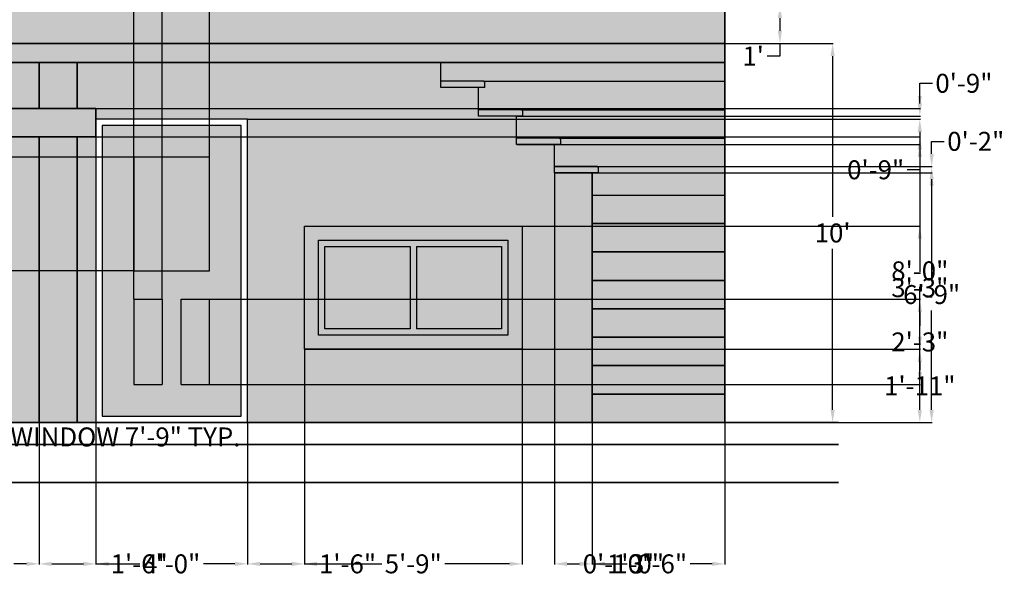
# Model space of a CAD drawing. Units: inches. Extents: x 23 to 640, y 58 to 516.
# Tile 3 of 4: x 328 to 640, y 67 to 243. Entities that reach past the tile are written whole.
import ezdxf

# ---------------------------------------------------------------- set-up
doc = ezdxf.new("R2010")
doc.units = ezdxf.units.IN
doc.header["$MEASUREMENT"] = 0
for name, color, linetype, lineweight in [('A-ANNO-DIMS', 2, 'Continuous', 18), ('A-DOOR', 3, 'Continuous', 25), ('A-ELEV', 7, 'Continuous', 35), ('A-ELEV-PATT', 252, 'Continuous', 13), ('A-FLOR-STRS', 7, 'Continuous', 25), ('A-GLAZ', 4, 'Continuous', 25)]:
    doc.layers.add(name, color=color, linetype=linetype, lineweight=lineweight)
doc.styles.get("Standard").update_dxf_attribs({"font": 'arial.ttf'})
doc.dimstyles.get("Standard").update_dxf_attribs({"dimtxt": 6, "dimasz": 4, "dimexe": 0.18, "dimexo": 0.0625, "dimgap": 2, "dimtad": 0, "dimtih": 1, "dimtoh": 1, "dimdec": 0, "dimzin": 0, "dimdsep": 46, "dimlunit": 3, "dimtxsty": 'Standard', "dimcen": 2, "dimadec": 0, "dimazin": 0, "dimtfac": 1, "dimtdec": 0, "dimtofl": 0, "dimtmove": 0, "dimatfit": 3, "dimfxl": 1, "dimtolj": 1, "dimtzin": 0, "dimarcsym": 0})

# ---------------------------------------------------------------- blocks, each defined once
blk = doc.blocks.new('*D9')
at = {"layer": 'A-ANNO-DIMS', "color": 0, "lineweight": -2, "transparency": 16777216}
for p, q in [((551.19, 247.68), (568.75, 247.68)), ((568.57, 243.68), (568.57, 239.68)), ((551.19, 235.68), (568.75, 235.68)), ((568.57, 235.68), (568.57, 231.68)), ((568.57, 231.68), (564.57, 231.68))]:
    blk.add_line(p, q, dxfattribs=at)
at = {"layer": 'A-ANNO-DIMS', "color": 0, "transparency": 16777216}
for points in [[(567.9, 243.68), (569.23, 243.68), (568.57, 247.68)], [(567.9, 239.68), (569.23, 239.68), (568.57, 235.68)]]:
    blk.add_solid(points, dxfattribs=at)
at = {"layer": 'Defpoints', "color": 0, "transparency": 16777216}
for p in [(551.13, 247.68), (551.13, 235.68), (568.57, 235.68)]:
    blk.add_point(p, dxfattribs=at)
at = {"layer": 'A-ANNO-DIMS', "color": 0, "transparency": 16777216, "insert": (560.09, 231.68), "char_height": 6, "attachment_point": 5}
blk.add_mtext("\\A1;1'", dxfattribs=at)
blk = doc.blocks.new('*D10')
at = {"layer": 'A-ANNO-DIMS', "color": 0, "lineweight": -2, "transparency": 16777216}
for p, q in [((551.19, 235.68), (585.45, 235.68)), ((585.27, 231.68), (585.27, 180.74)), ((585.27, 119.68), (585.27, 170.62)), ((551.19, 115.68), (585.45, 115.68))]:
    blk.add_line(p, q, dxfattribs=at)
at = {"layer": 'A-ANNO-DIMS', "color": 0, "transparency": 16777216}
for points in [[(584.6, 231.68), (585.93, 231.68), (585.27, 235.68)], [(584.6, 119.68), (585.93, 119.68), (585.27, 115.68)]]:
    blk.add_solid(points, dxfattribs=at)
at = {"layer": 'Defpoints', "color": 0, "transparency": 16777216}
for p in [(551.13, 235.68), (551.13, 115.68), (585.27, 115.68)]:
    blk.add_point(p, dxfattribs=at)
at = {"layer": 'A-ANNO-DIMS', "color": 0, "transparency": 16777216, "insert": (585.27, 175.68), "char_height": 6, "attachment_point": 5}
blk.add_mtext("\\A1;10'", dxfattribs=at)
blk = doc.blocks.new('*D15')
at = {"layer": 'A-ANNO-DIMS', "color": 0, "lineweight": -2, "transparency": 16777216}
for p, q in [((189.93, 125), (189.93, 110.93)), ((282.93, 125), (282.93, 110.93)), ((193.93, 111.11), (278.93, 111.11)), ((282.93, 111.11), (286.93, 111.11))]:
    blk.add_line(p, q, dxfattribs=at)
at = {"layer": 'A-ANNO-DIMS', "color": 0, "transparency": 16777216}
for points in [[(193.93, 111.78), (193.93, 110.44), (189.93, 111.11)], [(278.93, 111.78), (278.93, 110.44), (282.93, 111.11)]]:
    blk.add_solid(points, dxfattribs=at)
at = {"layer": 'Defpoints', "color": 0, "transparency": 16777216}
for p in [(189.93, 125.06), (282.93, 125.06), (282.93, 111.11)]:
    blk.add_point(p, dxfattribs=at)
at = {"layer": 'A-ANNO-DIMS', "color": 0, "transparency": 16777216, "insert": (344.69, 111.11), "char_height": 6, "attachment_point": 5}
blk.add_mtext('\\A1;SLIDING WINDOW 7\'-9" TYP.', dxfattribs=at)
blk = doc.blocks.new('*D26')
at = {"layer": 'A-ANNO-DIMS', "color": 0, "lineweight": -2, "transparency": 16777216}
for p, q in [((297.93, 115.62), (297.93, 70.75)), ((333.93, 115.62), (333.93, 70.75)), ((301.93, 70.93), (305.96, 70.93)), ((329.93, 70.93), (325.9, 70.93))]:
    blk.add_line(p, q, dxfattribs=at)
at = {"layer": 'A-ANNO-DIMS', "color": 0, "transparency": 16777216}
for points in [[(301.93, 71.6), (301.93, 70.26), (297.93, 70.93)], [(329.93, 71.6), (329.93, 70.26), (333.93, 70.93)]]:
    blk.add_solid(points, dxfattribs=at)
at = {"layer": 'Defpoints', "color": 0, "transparency": 16777216}
for p in [(297.93, 115.68), (333.93, 115.68), (333.93, 70.93)]:
    blk.add_point(p, dxfattribs=at)
at = {"layer": 'A-ANNO-DIMS', "color": 0, "transparency": 16777216, "insert": (315.93, 70.93), "char_height": 6, "attachment_point": 5}
blk.add_mtext('\\A1;3\'-0"', dxfattribs=at)
blk = doc.blocks.new('*D27')
at = {"layer": 'A-ANNO-DIMS', "color": 0, "lineweight": -2, "transparency": 16777216}
for p, q in [((333.93, 115.62), (333.93, 70.75)), ((351.93, 115.62), (351.93, 70.75)), ((337.93, 70.93), (347.93, 70.93)), ((351.93, 70.93), (355.93, 70.93))]:
    blk.add_line(p, q, dxfattribs=at)
at = {"layer": 'A-ANNO-DIMS', "color": 0, "transparency": 16777216}
for points in [[(337.93, 71.6), (337.93, 70.26), (333.93, 70.93)], [(347.93, 71.6), (347.93, 70.26), (351.93, 70.93)]]:
    blk.add_solid(points, dxfattribs=at)
at = {"layer": 'Defpoints', "color": 0, "transparency": 16777216}
for p in [(333.93, 115.68), (351.93, 115.68), (351.93, 70.93)]:
    blk.add_point(p, dxfattribs=at)
at = {"layer": 'A-ANNO-DIMS', "color": 0, "transparency": 16777216, "insert": (365.62, 70.93), "char_height": 6, "attachment_point": 5}
blk.add_mtext('\\A1;1\'-6"', dxfattribs=at)
blk = doc.blocks.new('*D28')
at = {"layer": 'A-ANNO-DIMS', "color": 0, "lineweight": -2, "transparency": 16777216}
for p, q in [((351.93, 115.62), (351.93, 70.75)), ((399.93, 115.62), (399.93, 70.75)), ((355.93, 70.93), (365.83, 70.93)), ((395.93, 70.93), (386.02, 70.93))]:
    blk.add_line(p, q, dxfattribs=at)
at = {"layer": 'A-ANNO-DIMS', "color": 0, "transparency": 16777216}
for points in [[(355.93, 71.6), (355.93, 70.26), (351.93, 70.93)], [(395.93, 71.6), (395.93, 70.26), (399.93, 70.93)]]:
    blk.add_solid(points, dxfattribs=at)
at = {"layer": 'Defpoints', "color": 0, "transparency": 16777216}
for p in [(351.93, 115.68), (399.93, 115.68), (399.93, 70.93)]:
    blk.add_point(p, dxfattribs=at)
at = {"layer": 'A-ANNO-DIMS', "color": 0, "transparency": 16777216, "insert": (375.93, 70.93), "char_height": 6, "attachment_point": 5}
blk.add_mtext('\\A1;4\'-0"', dxfattribs=at)
blk = doc.blocks.new('*D29')
at = {"layer": 'A-ANNO-DIMS', "color": 0, "lineweight": -2, "transparency": 16777216}
for p, q in [((417.93, 138.79), (417.93, 70.75)), ((399.93, 115.62), (399.93, 70.75)), ((403.93, 70.93), (413.93, 70.93)), ((417.93, 70.93), (421.93, 70.93))]:
    blk.add_line(p, q, dxfattribs=at)
at = {"layer": 'A-ANNO-DIMS', "color": 0, "transparency": 16777216}
for points in [[(403.93, 71.6), (403.93, 70.26), (399.93, 70.93)], [(413.93, 71.6), (413.93, 70.26), (417.93, 70.93)]]:
    blk.add_solid(points, dxfattribs=at)
at = {"layer": 'Defpoints', "color": 0, "transparency": 16777216}
for p in [(417.93, 138.86), (399.93, 115.68), (417.93, 70.93)]:
    blk.add_point(p, dxfattribs=at)
at = {"layer": 'A-ANNO-DIMS', "color": 0, "transparency": 16777216, "insert": (431.62, 70.93), "char_height": 6, "attachment_point": 5}
blk.add_mtext('\\A1;1\'-6"', dxfattribs=at)
blk = doc.blocks.new('*D30')
at = {"layer": 'A-ANNO-DIMS', "color": 0, "lineweight": -2, "transparency": 16777216}
for p, q in [((417.93, 138.79), (417.93, 70.75)), ((486.93, 138.79), (486.93, 70.75)), ((421.93, 70.93), (442.45, 70.93)), ((482.93, 70.93), (462.4, 70.93))]:
    blk.add_line(p, q, dxfattribs=at)
at = {"layer": 'A-ANNO-DIMS', "color": 0, "transparency": 16777216}
for points in [[(421.93, 71.6), (421.93, 70.26), (417.93, 70.93)], [(482.93, 71.6), (482.93, 70.26), (486.93, 70.93)]]:
    blk.add_solid(points, dxfattribs=at)
at = {"layer": 'Defpoints', "color": 0, "transparency": 16777216}
for p in [(417.93, 138.86), (486.93, 138.86), (486.93, 70.93)]:
    blk.add_point(p, dxfattribs=at)
at = {"layer": 'A-ANNO-DIMS', "color": 0, "transparency": 16777216, "insert": (452.43, 70.93), "char_height": 6, "attachment_point": 5}
blk.add_mtext('\\A1;5\'-9"', dxfattribs=at)
blk = doc.blocks.new('*D31')
at = {"layer": 'A-ANNO-DIMS', "color": 0, "lineweight": -2, "transparency": 16777216}
for p, q in [((497.13, 194.62), (497.13, 70.75)), ((486.93, 138.79), (486.93, 70.75)), ((482.93, 70.93), (478.93, 70.93)), ((501.13, 70.93), (505.13, 70.93))]:
    blk.add_line(p, q, dxfattribs=at)
at = {"layer": 'A-ANNO-DIMS', "color": 0, "transparency": 16777216}
for points in [[(482.93, 71.6), (482.93, 70.26), (486.93, 70.93)], [(501.13, 71.6), (501.13, 70.26), (497.13, 70.93)]]:
    blk.add_solid(points, dxfattribs=at)
at = {"layer": 'Defpoints', "color": 0, "transparency": 16777216}
for p in [(497.13, 194.68), (486.93, 138.86), (497.13, 70.93)]:
    blk.add_point(p, dxfattribs=at)
at = {"layer": 'A-ANNO-DIMS', "color": 0, "transparency": 16777216, "insert": (517.43, 70.93), "char_height": 6, "attachment_point": 5}
blk.add_mtext('\\A1;0\'-10"', dxfattribs=at)
blk = doc.blocks.new('*D32')
at = {"layer": 'A-ANNO-DIMS', "color": 0, "lineweight": -2, "transparency": 16777216}
for p, q in [((497.13, 194.62), (497.13, 70.75)), ((509.13, 194.62), (509.13, 70.75)), ((501.13, 70.93), (505.13, 70.93)), ((509.13, 70.93), (513.13, 70.93))]:
    blk.add_line(p, q, dxfattribs=at)
at = {"layer": 'A-ANNO-DIMS', "color": 0, "transparency": 16777216}
for points in [[(501.13, 71.6), (501.13, 70.26), (497.13, 70.93)], [(505.13, 71.6), (505.13, 70.26), (509.13, 70.93)]]:
    blk.add_solid(points, dxfattribs=at)
at = {"layer": 'Defpoints', "color": 0, "transparency": 16777216}
for p in [(497.13, 194.68), (509.13, 194.68), (509.13, 70.93)]:
    blk.add_point(p, dxfattribs=at)
at = {"layer": 'A-ANNO-DIMS', "color": 0, "transparency": 16777216, "insert": (522.82, 70.93), "char_height": 6, "attachment_point": 5}
blk.add_mtext('\\A1;1\'-0"', dxfattribs=at)
blk = doc.blocks.new('*D33')
at = {"layer": 'A-ANNO-DIMS', "color": 0, "lineweight": -2, "transparency": 16777216}
for p, q in [((509.13, 115.62), (509.13, 70.75)), ((551.13, 115.62), (551.13, 70.75)), ((513.13, 70.93), (520.16, 70.93)), ((547.13, 70.93), (540.1, 70.93))]:
    blk.add_line(p, q, dxfattribs=at)
at = {"layer": 'A-ANNO-DIMS', "color": 0, "transparency": 16777216}
for points in [[(513.13, 71.6), (513.13, 70.26), (509.13, 70.93)], [(547.13, 71.6), (547.13, 70.26), (551.13, 70.93)]]:
    blk.add_solid(points, dxfattribs=at)
at = {"layer": 'Defpoints', "color": 0, "transparency": 16777216}
for p in [(509.13, 115.68), (551.13, 115.68), (551.13, 70.93)]:
    blk.add_point(p, dxfattribs=at)
at = {"layer": 'A-ANNO-DIMS', "color": 0, "transparency": 16777216, "insert": (530.13, 70.93), "char_height": 6, "attachment_point": 5}
blk.add_mtext('\\A1;3\'-6"', dxfattribs=at)
blk = doc.blocks.new('*D35')
at = {"layer": 'A-ANNO-DIMS', "color": 0, "lineweight": -2, "transparency": 16777216}
for p, q in [((399.99, 211.68), (613.06, 211.68)), ((612.88, 207.68), (612.88, 168.74)), ((612.88, 119.68), (612.88, 158.62)), ((399.99, 115.68), (613.06, 115.68))]:
    blk.add_line(p, q, dxfattribs=at)
at = {"layer": 'A-ANNO-DIMS', "color": 0, "transparency": 16777216}
for points in [[(612.21, 207.68), (613.55, 207.68), (612.88, 211.68)], [(612.21, 119.68), (613.55, 119.68), (612.88, 115.68)]]:
    blk.add_solid(points, dxfattribs=at)
at = {"layer": 'Defpoints', "color": 0, "transparency": 16777216}
for p in [(399.93, 211.68), (612.88, 211.68), (399.93, 115.68)]:
    blk.add_point(p, dxfattribs=at)
at = {"layer": 'A-ANNO-DIMS', "color": 0, "transparency": 16777216, "insert": (612.88, 163.68), "char_height": 6, "attachment_point": 5}
blk.add_mtext('\\A1;8\'-0"', dxfattribs=at)
blk = doc.blocks.new('*D36')
at = {"layer": 'A-ANNO-DIMS', "color": 0, "lineweight": -2, "transparency": 16777216}
for p, q in [((359.93, 507.43), (355.93, 507.43)), ((363.93, 163.74), (363.93, 507.61)), ((387.93, 199.74), (387.93, 507.61)), ((391.93, 507.43), (395.93, 507.43))]:
    blk.add_line(p, q, dxfattribs=at)
at = {"layer": 'A-ANNO-DIMS', "color": 0, "transparency": 16777216}
for points in [[(359.93, 508.1), (359.93, 506.76), (363.93, 507.43)], [(391.93, 508.1), (391.93, 506.76), (387.93, 507.43)]]:
    blk.add_solid(points, dxfattribs=at)
at = {"layer": 'Defpoints', "color": 0, "transparency": 16777216}
for p in [(387.93, 507.43), (387.93, 199.68), (363.93, 163.68)]:
    blk.add_point(p, dxfattribs=at)
at = {"layer": 'A-ANNO-DIMS', "color": 0, "transparency": 16777216, "insert": (375.93, 507.43), "char_height": 6, "attachment_point": 5}
blk.add_mtext('\\A1;2\'-0"', dxfattribs=at)
blk = doc.blocks.new('*D37')
at = {"layer": 'A-ANNO-DIMS', "color": 0, "lineweight": -2, "transparency": 16777216}
for p, q in [((363.87, 199.68), (63.5, 199.68)), ((63.68, 195.68), (63.68, 186.75)), ((63.68, 167.68), (63.68, 176.62)), ((363.87, 163.68), (63.5, 163.68))]:
    blk.add_line(p, q, dxfattribs=at)
at = {"layer": 'A-ANNO-DIMS', "color": 0, "transparency": 16777216}
for points in [[(63.01, 195.68), (64.35, 195.68), (63.68, 199.68)], [(63.01, 167.68), (64.35, 167.68), (63.68, 163.68)]]:
    blk.add_solid(points, dxfattribs=at)
at = {"layer": 'Defpoints', "color": 0, "transparency": 16777216}
for p in [(63.68, 199.68), (363.93, 199.68), (363.93, 163.68)]:
    blk.add_point(p, dxfattribs=at)
at = {"layer": 'A-ANNO-DIMS', "color": 0, "transparency": 16777216, "insert": (63.68, 181.68), "char_height": 6, "attachment_point": 5}
blk.add_mtext('\\A1;3\'-0"', dxfattribs=at)
blk = doc.blocks.new('*D38')
at = {"layer": 'A-ANNO-DIMS', "color": 0, "lineweight": -2, "transparency": 16777216}
for p, q in [((359.93, 507.43), (355.93, 507.43)), ((363.93, 154.74), (363.93, 507.61)), ((372.93, 154.74), (372.93, 507.61)), ((376.93, 507.43), (380.93, 507.43))]:
    blk.add_line(p, q, dxfattribs=at)
at = {"layer": 'A-ANNO-DIMS', "color": 0, "transparency": 16777216}
for points in [[(359.93, 508.1), (359.93, 506.76), (363.93, 507.43)], [(376.93, 508.1), (376.93, 506.76), (372.93, 507.43)]]:
    blk.add_solid(points, dxfattribs=at)
at = {"layer": 'Defpoints', "color": 0, "transparency": 16777216}
for p in [(372.93, 507.43), (363.93, 154.68), (372.93, 154.68)]:
    blk.add_point(p, dxfattribs=at)
at = {"layer": 'A-ANNO-DIMS', "color": 0, "transparency": 16777216, "insert": (390.9, 507.43), "char_height": 6, "attachment_point": 5}
blk.add_mtext('\\A1;0\'-9"', dxfattribs=at)
blk = doc.blocks.new('*D39')
at = {"layer": 'A-ANNO-DIMS', "color": 0, "lineweight": -2, "transparency": 16777216}
for p, q in [((387.99, 154.68), (613.06, 154.68)), ((612.88, 150.68), (612.88, 146.25)), ((612.88, 131.68), (612.88, 136.12)), ((387.99, 127.68), (613.06, 127.68))]:
    blk.add_line(p, q, dxfattribs=at)
at = {"layer": 'A-ANNO-DIMS', "color": 0, "transparency": 16777216}
for points in [[(612.21, 150.68), (613.55, 150.68), (612.88, 154.68)], [(612.21, 131.68), (613.55, 131.68), (612.88, 127.68)]]:
    blk.add_solid(points, dxfattribs=at)
at = {"layer": 'Defpoints', "color": 0, "transparency": 16777216}
for p in [(387.93, 154.68), (612.88, 154.68), (387.93, 127.68)]:
    blk.add_point(p, dxfattribs=at)
at = {"layer": 'A-ANNO-DIMS', "color": 0, "transparency": 16777216, "insert": (612.88, 141.18), "char_height": 6, "attachment_point": 5}
blk.add_mtext('\\A1;2\'-3"', dxfattribs=at)
blk = doc.blocks.new('*D40')
at = {"layer": 'A-ANNO-DIMS', "color": 0, "lineweight": -2, "transparency": 16777216}
for p, q in [((417.99, 138.86), (613.06, 138.86)), ((612.88, 134.86), (612.88, 132.28)), ((612.88, 119.68), (612.88, 122.26)), ((399.99, 115.68), (613.06, 115.68))]:
    blk.add_line(p, q, dxfattribs=at)
at = {"layer": 'A-ANNO-DIMS', "color": 0, "transparency": 16777216}
for points in [[(612.21, 134.86), (613.55, 134.86), (612.88, 138.86)], [(612.21, 119.68), (613.55, 119.68), (612.88, 115.68)]]:
    blk.add_solid(points, dxfattribs=at)
at = {"layer": 'Defpoints', "color": 0, "transparency": 16777216}
for p in [(417.93, 138.86), (612.88, 138.86), (399.93, 115.68)]:
    blk.add_point(p, dxfattribs=at)
at = {"layer": 'A-ANNO-DIMS', "color": 0, "transparency": 16777216, "insert": (612.88, 127.27), "char_height": 6, "attachment_point": 5}
blk.add_mtext('\\A1;1\'-11"', dxfattribs=at)
blk = doc.blocks.new('*D41')
at = {"layer": 'A-ANNO-DIMS', "color": 0, "lineweight": -2, "transparency": 16777216}
for p, q in [((486.99, 177.86), (613.06, 177.86)), ((612.88, 173.86), (612.88, 163.42)), ((612.88, 142.86), (612.88, 153.29)), ((486.99, 138.86), (613.06, 138.86))]:
    blk.add_line(p, q, dxfattribs=at)
at = {"layer": 'A-ANNO-DIMS', "color": 0, "transparency": 16777216}
for points in [[(612.21, 173.86), (613.55, 173.86), (612.88, 177.86)], [(612.21, 142.86), (613.55, 142.86), (612.88, 138.86)]]:
    blk.add_solid(points, dxfattribs=at)
at = {"layer": 'Defpoints', "color": 0, "transparency": 16777216}
for p in [(486.93, 177.86), (612.88, 177.86), (486.93, 138.86)]:
    blk.add_point(p, dxfattribs=at)
at = {"layer": 'A-ANNO-DIMS', "color": 0, "transparency": 16777216, "insert": (612.88, 158.36), "char_height": 6, "attachment_point": 5}
blk.add_mtext('\\A1;3\'-3"', dxfattribs=at)
blk = doc.blocks.new('*D46')
at = {"layer": 'A-ANNO-DIMS', "color": 0, "lineweight": -2, "transparency": 16777216}
for p, q in [((612.88, 216.68), (612.88, 220.68)), ((485.19, 212.68), (613.06, 212.68)), ((485.19, 203.68), (613.06, 203.68)), ((612.88, 199.68), (612.88, 195.68)), ((612.88, 195.68), (608.88, 195.68))]:
    blk.add_line(p, q, dxfattribs=at)
at = {"layer": 'A-ANNO-DIMS', "color": 0, "transparency": 16777216}
for points in [[(612.21, 216.68), (613.55, 216.68), (612.88, 212.68)], [(612.21, 199.68), (613.55, 199.68), (612.88, 203.68)]]:
    blk.add_solid(points, dxfattribs=at)
at = {"layer": 'Defpoints', "color": 0, "transparency": 16777216}
for p in [(485.13, 212.68), (485.13, 203.68), (612.88, 203.68)]:
    blk.add_point(p, dxfattribs=at)
at = {"layer": 'A-ANNO-DIMS', "color": 0, "transparency": 16777216, "insert": (598.9, 195.68), "char_height": 6, "attachment_point": 5}
blk.add_mtext('\\A1;0\'-9"', dxfattribs=at)
blk = doc.blocks.new('*D47')
at = {"layer": 'A-ANNO-DIMS', "color": 0, "lineweight": -2, "transparency": 16777216}
for p, q in [((612.88, 219.06), (612.88, 223.06)), ((612.88, 223.06), (616.88, 223.06)), ((351.99, 215.06), (613.06, 215.06)), ((351.99, 206.06), (613.06, 206.06)), ((612.88, 202.06), (612.88, 198.06))]:
    blk.add_line(p, q, dxfattribs=at)
at = {"layer": 'A-ANNO-DIMS', "color": 0, "transparency": 16777216}
for points in [[(612.21, 219.06), (613.55, 219.06), (612.88, 215.06)], [(612.21, 202.06), (613.55, 202.06), (612.88, 206.06)]]:
    blk.add_solid(points, dxfattribs=at)
at = {"layer": 'Defpoints', "color": 0, "transparency": 16777216}
for p in [(351.93, 215.06), (612.88, 215.06), (351.93, 206.06)]:
    blk.add_point(p, dxfattribs=at)
at = {"layer": 'A-ANNO-DIMS', "color": 0, "transparency": 16777216, "insert": (626.85, 223.06), "char_height": 6, "attachment_point": 5}
blk.add_mtext('\\A1;0\'-9"', dxfattribs=at)
blk = doc.blocks.new('*D50')
at = {"layer": 'A-ANNO-DIMS', "color": 0, "lineweight": -2, "transparency": 16777216}
for p, q in [((510.69, 196.68), (616.81, 196.68)), ((616.63, 192.68), (616.63, 161.24)), ((616.63, 119.68), (616.63, 151.12)), ((509.19, 115.68), (616.81, 115.68))]:
    blk.add_line(p, q, dxfattribs=at)
at = {"layer": 'A-ANNO-DIMS', "color": 0, "transparency": 16777216}
for points in [[(615.96, 192.68), (617.3, 192.68), (616.63, 196.68)], [(615.96, 119.68), (617.3, 119.68), (616.63, 115.68)]]:
    blk.add_solid(points, dxfattribs=at)
at = {"layer": 'Defpoints', "color": 0, "transparency": 16777216}
for p in [(510.63, 196.68), (616.63, 196.68), (509.13, 115.68)]:
    blk.add_point(p, dxfattribs=at)
at = {"layer": 'A-ANNO-DIMS', "color": 0, "transparency": 16777216, "insert": (616.63, 156.18), "char_height": 6, "attachment_point": 5}
blk.add_mtext('\\A1;6\'-9"', dxfattribs=at)
blk = doc.blocks.new('*D51')
at = {"layer": 'A-ANNO-DIMS', "color": 0, "lineweight": -2, "transparency": 16777216}
for p, q in [((616.63, 200.68), (616.63, 204.68)), ((616.63, 204.68), (620.63, 204.68)), ((497.19, 196.68), (616.81, 196.68)), ((497.19, 194.68), (616.81, 194.68)), ((616.63, 190.68), (616.63, 186.68))]:
    blk.add_line(p, q, dxfattribs=at)
at = {"layer": 'A-ANNO-DIMS', "color": 0, "transparency": 16777216}
for points in [[(615.96, 200.68), (617.3, 200.68), (616.63, 196.68)], [(615.96, 190.68), (617.3, 190.68), (616.63, 194.68)]]:
    blk.add_solid(points, dxfattribs=at)
at = {"layer": 'Defpoints', "color": 0, "transparency": 16777216}
for p in [(497.13, 196.68), (616.63, 196.68), (497.13, 194.68)]:
    blk.add_point(p, dxfattribs=at)
at = {"layer": 'A-ANNO-DIMS', "color": 0, "transparency": 16777216, "insert": (630.6, 204.68), "char_height": 6, "attachment_point": 5}
blk.add_mtext('\\A1;0\'-2"', dxfattribs=at)

msp = doc.modelspace()

# ---------------------------------------------------------------- hatches: boundary and pattern name
at = {"layer": 'A-ELEV-PATT'}
h = msp.add_hatch(color=256, dxfattribs=at)
h.dxf.hatch_style = 1
h.paths.add_polyline_path([(333.93, 433.68), (297.93, 433.68), (297.93, 379.68), (333.93, 379.68)])
h.paths.add_polyline_path([(333.93, 379.68), (297.93, 379.68), (297.93, 367.68), (333.93, 367.68)])
h.paths.add_polyline_path([(333.93, 358.68), (297.93, 358.68), (297.93, 247.68), (333.93, 247.68)])
h.paths.add_polyline_path([(333.93, 229.68), (297.93, 229.68), (297.93, 215.06), (333.93, 215.06)])
h.paths.add_polyline_path([(333.93, 206.06), (297.93, 206.06), (297.93, 115.68), (333.93, 115.68)])
h = msp.add_hatch(color=256, dxfattribs=at)
h.dxf.hatch_style = 1
h.paths.add_polyline_path([(371.93, 367.68), (180.93, 367.68), (180.93, 247.68), (189.93, 247.68), (189.93, 358.68), (371.93, 358.68)])
h.paths.add_polyline_path([(189.93, 247.68), (180.93, 247.68), (180.93, 235.68), (189.93, 235.68)])
h.paths.add_polyline_path([(189.93, 235.68), (180.93, 235.68), (180.93, 206.06), (333.93, 206.06), (351.93, 206.06), (351.93, 211.68), (351.93, 215.06), (189.93, 215.06)])
h.paths.add_polyline_path([(551.13, 247.68), (280.13, 247.68), (280.13, 235.68), (551.13, 235.68)])
h.paths.add_polyline_path([(551.13, 235.68), (280.13, 235.68), (280.13, 229.68), (551.13, 229.68)])
h = msp.add_hatch(color=256, dxfattribs=at)
h.set_gradient(color1=(147, 149, 152), color2=(199, 200, 202), name='INVCYLINDER')
h.paths.add_polyline_path([(333.93, 215.06), (345.93, 215.06), (345.93, 229.68), (333.93, 229.68)])
h = msp.add_hatch(color=256, dxfattribs=at)
h.set_gradient(color1=(255, 255, 255), color2=(147, 149, 152), name='INVHEMISPHERICAL')
h.paths.add_polyline_path([(399.93, 115.68), (509.13, 115.68), (509.13, 187.68), (509.13, 194.68), (497.13, 194.68), (497.13, 203.68), (485.13, 203.68), (485.13, 212.68), (473.13, 212.68), (473.13, 221.68), (461.13, 221.68), (461.13, 229.68), (345.93, 229.68), (345.93, 215.06), (351.93, 215.06), (351.93, 211.68), (399.93, 211.68)])
h.paths.add_polyline_path([(486.93, 177.86), (486.93, 138.86), (417.93, 138.86), (417.93, 177.86)], flags=16)
h.paths.add_polyline_path([(482.43, 173.36), (482.43, 143.36), (422.43, 143.36), (422.43, 173.36)], flags=0)
h.paths.add_polyline_path([(451.43, 171.36), (451.43, 145.36), (424.43, 145.36), (424.43, 171.36)], flags=0)
h.paths.add_polyline_path([(453.43, 171.36), (480.43, 171.36), (480.43, 145.36), (453.43, 145.36)], flags=0)
h = msp.add_hatch(color=256, dxfattribs=at)
h.set_gradient(color1=(206, 204, 230), color2=(99, 100, 102), name='INVHEMISPHERICAL')
h.paths.add_polyline_path([(551.13, 229.68), (461.13, 229.68), (461.13, 223.68), (474.63, 223.68), (551.13, 223.68)])
h.paths.add_polyline_path([(551.13, 223.68), (474.63, 223.68, -0.414214), (475.13, 223.18), (475.13, 221.68), (473.13, 221.68), (473.13, 214.68), (486.63, 214.68), (551.13, 214.68)])
h.paths.add_polyline_path([(551.13, 214.68), (486.63, 214.68, -0.414214), (487.13, 214.18), (487.13, 212.68), (485.13, 212.68), (485.13, 205.68), (498.63, 205.68), (551.13, 205.68)])
h.paths.add_polyline_path([(551.13, 205.68), (498.63, 205.68, -0.414214), (499.13, 205.18), (499.13, 203.68), (497.13, 203.68), (497.13, 196.68), (510.63, 196.68), (551.13, 196.68)])
h.paths.add_polyline_path([(551.13, 196.68), (510.63, 196.68, -0.414214), (511.13, 196.18), (511.13, 194.68), (509.13, 194.68), (509.13, 187.68), (551.13, 187.68)])
h = msp.add_hatch(color=256, dxfattribs=at)
h.set_gradient(color1=(255, 255, 255), color2=(147, 149, 152))
h.paths.add_polyline_path([(461.13, 223.68), (461.13, 221.68), (475.13, 221.68), (475.13, 223.18, 0.414214), (474.63, 223.68)])
h.paths.add_polyline_path([(487.13, 212.68), (487.13, 214.18, 0.414214), (486.63, 214.68), (473.13, 214.68), (473.13, 212.68)])
h.paths.add_polyline_path([(499.13, 203.68), (499.13, 205.18, 0.414214), (498.63, 205.68), (485.13, 205.68), (485.13, 203.68)])
h.paths.add_polyline_path([(497.13, 196.68), (497.13, 194.68), (511.13, 194.68), (511.13, 196.18, 0.414214), (510.63, 196.68)])
h = msp.add_hatch(color=256, dxfattribs=at)
h.set_gradient(color1=(255, 255, 255), color2=(147, 149, 152), name='SPHERICAL')
h.paths.add_polyline_path([(353.93, 117.68), (397.93, 117.68), (397.93, 209.68), (353.93, 209.68)])
h.paths.add_polyline_path([(363.93, 163.68), (363.93, 199.68), (387.93, 199.68), (387.93, 163.68)], flags=16)
h.paths.add_polyline_path([(363.93, 154.68), (372.93, 154.68), (372.93, 127.68), (363.93, 127.68)], flags=16)
h.paths.add_polyline_path([(378.93, 154.68), (387.93, 154.68), (387.93, 127.68), (378.93, 127.68)], flags=16)
h = msp.add_hatch(color=256, dxfattribs=at)
h.set_gradient(color1=(147, 149, 152), color2=(199, 200, 202), name='INVCYLINDER')
h.paths.add_polyline_path([(345.93, 206.06), (333.93, 206.06), (333.93, 115.68), (345.93, 115.68)])
h = msp.add_hatch(color=256, dxfattribs=at)
h.set_gradient(color1=(255, 255, 255), color2=(147, 149, 152), name='CYLINDER')
h.paths.add_polyline_path([(345.93, 115.68), (351.93, 115.68), (351.93, 206.06), (345.93, 206.06)])
h = msp.add_hatch(color=256, dxfattribs=at)
h.set_gradient(color1=(99, 100, 102), color2=(147, 149, 152), name='CYLINDER')
h.paths.add_polyline_path([(363.93, 163.68), (387.93, 163.68), (387.93, 199.68), (363.93, 199.68)])
h = msp.add_hatch(color=256, dxfattribs=at)
h.set_gradient(color1=(199, 200, 202), color2=(147, 149, 152), name='CYLINDER')
h.paths.add_polyline_path([(509.13, 187.68), (509.13, 178.68), (551.13, 178.68), (551.13, 187.68)])
h = msp.add_hatch(color=256, dxfattribs=at)
h.set_gradient(color1=(153, 76, 76), color2=(147, 149, 152), name='SPHERICAL')
h.paths.add_polyline_path([(417.93, 177.86), (417.93, 138.86), (486.93, 138.86), (486.93, 177.86)])
h.paths.add_polyline_path([(422.43, 173.36), (482.43, 173.36), (482.43, 143.36), (422.43, 143.36)], flags=16)
h.paths.add_polyline_path([(424.43, 171.36), (451.43, 171.36), (451.43, 145.36), (424.43, 145.36)], flags=0)
h.paths.add_polyline_path([(453.43, 171.36), (480.43, 171.36), (480.43, 145.36), (453.43, 145.36)], flags=0)
h = msp.add_hatch(color=256, dxfattribs=at)
h.set_gradient(color1=(147, 149, 152), color2=(199, 200, 202), name='CYLINDER')
h.paths.add_polyline_path([(551.13, 169.68), (551.13, 178.68), (509.13, 178.68), (509.13, 169.68)])
h = msp.add_hatch(color=256, dxfattribs=at)
h.set_gradient(color1=(99, 100, 102), color2=(66, 66, 66), name='SPHERICAL')
h.paths.add_polyline_path([(422.43, 173.36), (422.43, 143.36), (482.43, 143.36), (482.43, 173.36)])
h.paths.add_polyline_path([(424.43, 171.36), (451.43, 171.36), (451.43, 145.36), (424.43, 145.36)], flags=16)
h.paths.add_polyline_path([(453.43, 171.36), (480.43, 171.36), (480.43, 145.36), (453.43, 145.36)], flags=16)
h = msp.add_hatch(color=256, dxfattribs=at)
h.set_gradient(color1=(255, 255, 255), color2=(173, 221, 247), name='INVSPHERICAL')
h.paths.add_polyline_path([(451.43, 171.36), (424.43, 171.36), (424.43, 145.36), (451.43, 145.36)])
h = msp.add_hatch(color=256, dxfattribs=at)
h.set_gradient(color1=(255, 255, 255), color2=(173, 221, 247), name='INVSPHERICAL')
h.paths.add_polyline_path([(480.43, 145.36), (480.43, 171.36), (453.43, 171.36), (453.43, 145.36)])
h = msp.add_hatch(color=256, dxfattribs=at)
h.set_gradient(color1=(199, 200, 202), color2=(147, 149, 152), name='CYLINDER')
h.paths.add_polyline_path([(509.13, 169.68), (509.13, 160.68), (551.13, 160.68), (551.13, 169.68)])
h = msp.add_hatch(color=256, dxfattribs=at)
h.set_gradient(color1=(147, 149, 152), color2=(199, 200, 202), name='CYLINDER')
h.paths.add_polyline_path([(509.13, 160.68), (509.13, 151.68), (551.13, 151.68), (551.13, 160.68)])
h = msp.add_hatch(color=256, dxfattribs=at)
h.set_gradient(color1=(99, 100, 102), color2=(147, 149, 152), name='CYLINDER')
h.paths.add_polyline_path([(372.93, 154.68), (363.93, 154.68), (363.93, 127.68), (372.93, 127.68)])
h = msp.add_hatch(color=256, dxfattribs=at)
h.set_gradient(color1=(99, 100, 102), color2=(147, 149, 152), name='CYLINDER')
h.paths.add_polyline_path([(378.93, 127.68), (387.93, 127.68), (387.93, 154.68), (378.93, 154.68)])
h = msp.add_hatch(color=256, dxfattribs=at)
h.set_gradient(color1=(199, 200, 202), color2=(147, 149, 152), name='CYLINDER')
h.paths.add_polyline_path([(551.13, 142.68), (551.13, 151.68), (509.13, 151.68), (509.13, 142.68)])
h = msp.add_hatch(color=256, dxfattribs=at)
h.set_gradient(color1=(147, 149, 152), color2=(199, 200, 202), name='CYLINDER')
h.paths.add_polyline_path([(509.13, 142.68), (509.13, 133.68), (551.13, 133.68), (551.13, 142.68)])
h = msp.add_hatch(color=256, dxfattribs=at)
h.set_gradient(color1=(199, 200, 202), color2=(147, 149, 152), name='CYLINDER')
h.paths.add_polyline_path([(551.13, 124.68), (551.13, 133.68), (509.13, 133.68), (509.13, 124.68)])
h = msp.add_hatch(color=256, dxfattribs=at)
h.set_gradient(color1=(147, 149, 152), color2=(199, 200, 202), name='CYLINDER')
h.paths.add_polyline_path([(509.13, 124.68), (509.13, 115.68), (551.13, 115.68), (551.13, 124.68)])

# ---------------------------------------------------------------- linework, layer by layer
at = {"layer": 'A-DOOR'}
for p, q in [((387.93, 199.68), (363.93, 199.68)), ((363.93, 199.68), (363.93, 163.68)), ((387.93, 163.68), (387.93, 199.68)), ((363.93, 163.68), (387.93, 163.68)), ((363.93, 154.68), (372.93, 154.68)), ((363.93, 154.68), (363.93, 127.68)), ((372.93, 154.68), (372.93, 127.68)), ((378.93, 127.68), (378.93, 154.68)), ((378.93, 154.68), (387.93, 154.68)), ((387.93, 127.68), (387.93, 154.68)), ((363.93, 127.68), (372.93, 127.68)), ((378.93, 127.68), (387.93, 127.68))]:
    msp.add_line(p, q, dxfattribs=at)
for points in [[(351.93, 115.68), (399.93, 115.68), (399.93, 211.68), (351.93, 211.68)], [(353.93, 117.68), (397.93, 117.68), (397.93, 209.68), (353.93, 209.68)]]:
    msp.add_lwpolyline(points, close=True, dxfattribs=at)
at = {"layer": 'A-ELEV'}
for p, q in [((551.13, 379.68), (551.13, 115.68)), ((125.43, 235.68), (551.13, 235.68)), ((280.13, 229.68), (551.13, 229.68)), ((333.93, 229.68), (333.93, 215.06)), ((345.93, 229.68), (345.93, 215.06)), ((351.93, 215.06), (189.93, 215.06)), ((351.93, 206.06), (351.93, 215.06)), ((180.93, 206.06), (333.93, 206.06)), ((333.93, 206.06), (351.93, 206.06)), ((333.93, 206.06), (333.93, 115.68)), ((345.93, 206.06), (345.93, 115.68)), ((509.13, 187.68), (509.13, 115.68)), ((509.13, 178.68), (551.13, 178.68)), ((509.13, 169.68), (551.13, 169.68)), ((509.13, 160.68), (551.13, 160.68)), ((509.13, 151.68), (551.13, 151.68)), ((509.13, 142.68), (551.13, 142.68)), ((509.13, 133.68), (551.13, 133.68)), ((509.13, 124.68), (551.13, 124.68)), ((89.43, 115.68), (587.13, 115.68)), ((89.43, 108.68), (587.13, 108.68)), ((89.43, 96.68), (587.13, 96.68))]:
    msp.add_line(p, q, dxfattribs=at)
at = {"layer": 'A-FLOR-STRS'}
for p, q in [((461.13, 221.68), (461.13, 229.68)), ((474.63, 223.68), (461.13, 223.68)), ((475.13, 221.68), (461.13, 221.68)), ((473.13, 212.68), (473.13, 221.68)), ((474.63, 223.68), (551.13, 223.68)), ((475.13, 221.68), (475.13, 223.18)), ((486.63, 214.68), (473.13, 214.68)), ((487.13, 212.68), (473.13, 212.68)), ((485.13, 203.68), (485.13, 212.68)), ((486.63, 214.68), (551.13, 214.68)), ((487.13, 212.68), (487.13, 214.18)), ((498.63, 205.68), (485.13, 205.68)), ((499.13, 203.68), (485.13, 203.68)), ((497.13, 194.68), (497.13, 203.68)), ((498.63, 205.68), (551.13, 205.68)), ((499.13, 203.68), (499.13, 205.18)), ((510.63, 196.68), (497.13, 196.68)), ((510.63, 196.68), (551.13, 196.68)), ((511.13, 194.68), (497.13, 194.68)), ((509.13, 187.68), (509.13, 194.68)), ((511.13, 194.68), (511.13, 196.18)), ((509.13, 187.68), (551.13, 187.68))]:
    msp.add_line(p, q, dxfattribs=at)
for centre in [(474.63, 223.18), (486.63, 214.18), (498.63, 205.18), (510.63, 196.18)]:
    msp.add_arc(centre, 0.5, 0, 90, dxfattribs=at)
at = {"layer": 'A-GLAZ'}
for p, q in [((451.43, 171.36), (451.43, 145.36)), ((453.43, 171.36), (453.43, 145.36))]:
    msp.add_line(p, q, dxfattribs=at)
for points in [[(417.93, 177.86), (486.93, 177.86), (486.93, 138.86), (417.93, 138.86)], [(422.43, 173.36), (482.43, 173.36), (482.43, 143.36), (422.43, 143.36)]]:
    msp.add_lwpolyline(points, close=True, dxfattribs=at)
for points in [[(451.43, 145.36), (424.43, 145.36), (424.43, 171.36), (451.43, 171.36)], [(453.43, 171.36), (480.43, 171.36), (480.43, 145.36), (453.43, 145.36)]]:
    msp.add_lwpolyline(points, dxfattribs=at)

# ---------------------------------------------------------------- dimensions: what is measured, and where the dimension line sits
at = {"layer": 'A-ANNO-DIMS'}
for base, p1, p2, picture, middle in [((387.93, 507.43), (363.93, 163.68), (387.93, 199.68), '*D36', (375.93, 507.43)), ((372.93, 507.43), (363.93, 154.68), (372.93, 154.68), '*D38', (390.9, 507.43)), ((497.13, 70.93), (486.93, 138.86), (497.13, 194.68), '*D31', (517.43, 70.93)), ((509.13, 70.93), (497.13, 194.68), (509.13, 194.68), '*D32', (522.82, 70.93)), ((417.93, 70.93), (399.93, 115.68), (417.93, 138.86), '*D29', (431.62, 70.93)), ((486.93, 70.93), (417.93, 138.86), (486.93, 138.86), '*D30', (452.43, 70.93)), ((333.93, 70.93), (297.93, 115.68), (333.93, 115.68), '*D26', (315.93, 70.93)), ((351.93, 70.93), (333.93, 115.68), (351.93, 115.68), '*D27', (365.62, 70.93)), ((399.93, 70.93), (351.93, 115.68), (399.93, 115.68), '*D28', (375.93, 70.93)), ((551.13, 70.93), (509.13, 115.68), (551.13, 115.68), '*D33', (530.13, 70.93))]:
    dim = msp.add_linear_dim(base=base, p1=p1, p2=p2, dimstyle='Standard', override={"dimdec": 1, "dimlfac": 1, "dimrnd": 0, "dimzin": 1, "dimdsep": 46, "dimlunit": 4, "dimfrac": 2}, dxfattribs=at)
    dim.commit()
    dim.dimension.update_dxf_attribs({"geometry": picture, "text_midpoint": middle})
for base, p1, p2, override, picture, middle in [((568.57, 235.68), (551.13, 247.68), (551.13, 235.68), {"dimclrd": 0, "dimclre": 0, "dimclrt": 0}, '*D9', (560.09, 231.68)), ((585.27, 115.68), (551.13, 235.68), (551.13, 115.68), {"dimclrd": 0, "dimclre": 0, "dimclrt": 0}, '*D10', (585.27, 175.68)), ((612.88, 215.06), (351.93, 206.06), (351.93, 215.06), {"dimdec": 1, "dimlfac": 1, "dimrnd": 0, "dimzin": 1, "dimdsep": 46, "dimlunit": 4, "dimfrac": 2}, '*D47', (626.85, 223.06)), ((612.88, 203.68), (485.13, 212.68), (485.13, 203.68), {"dimdec": 1, "dimlfac": 1, "dimrnd": 0, "dimzin": 1, "dimdsep": 46, "dimlunit": 4, "dimfrac": 2}, '*D46', (598.9, 195.68)), ((612.88, 211.68), (399.93, 115.68), (399.93, 211.68), {"dimdec": 1, "dimlfac": 1, "dimrnd": 0, "dimzin": 1, "dimdsep": 46, "dimlunit": 4, "dimfrac": 2}, '*D35', (612.88, 163.68)), ((616.63, 196.68), (497.13, 194.68), (497.13, 196.68), {"dimdec": 1, "dimlfac": 1, "dimrnd": 0, "dimzin": 1, "dimdsep": 46, "dimlunit": 4, "dimfrac": 2}, '*D51', (630.6, 204.68)), ((63.68, 199.68), (363.93, 163.68), (363.93, 199.68), {"dimdec": 1, "dimlfac": 1, "dimrnd": 0, "dimzin": 1, "dimdsep": 46, "dimlunit": 4, "dimfrac": 2}, '*D37', (63.68, 181.68)), ((616.63, 196.68), (509.13, 115.68), (510.63, 196.68), {"dimdec": 1, "dimlfac": 1, "dimrnd": 0, "dimzin": 1, "dimdsep": 46, "dimlunit": 4, "dimfrac": 2}, '*D50', (616.63, 156.18)), ((612.88, 177.86), (486.93, 138.86), (486.93, 177.86), {"dimdec": 1, "dimlfac": 1, "dimrnd": 0, "dimzin": 1, "dimdsep": 46, "dimlunit": 4, "dimfrac": 2}, '*D41', (612.88, 158.36)), ((612.88, 154.68), (387.93, 127.68), (387.93, 154.68), {"dimdec": 1, "dimlfac": 1, "dimrnd": 0, "dimzin": 1, "dimdsep": 46, "dimlunit": 4, "dimfrac": 2}, '*D39', (612.88, 141.18)), ((612.88, 138.86), (399.93, 115.68), (417.93, 138.86), {"dimdec": 1, "dimlfac": 1, "dimrnd": 0, "dimzin": 1, "dimdsep": 46, "dimlunit": 4, "dimfrac": 2}, '*D40', (612.88, 127.27))]:
    dim = msp.add_linear_dim(base=base, p1=p1, p2=p2, angle=90, dimstyle='Standard', override=override, dxfattribs=at)
    dim.commit()
    dim.dimension.update_dxf_attribs({"geometry": picture, "text_midpoint": middle})
dim = msp.add_linear_dim(base=(282.93, 111.11), p1=(189.93, 125.06), p2=(282.93, 125.06), text='SLIDING WINDOW <> TYP.', dimstyle='Standard', override={"dimdec": 1, "dimrnd": 0, "dimzin": 1, "dimlunit": 4, "dimfrac": 2}, dxfattribs=at)
dim.commit()
dim.dimension.update_dxf_attribs({"geometry": '*D15', "text_midpoint": (344.69, 111.11)})

doc.saveas('drawing.dxf')
